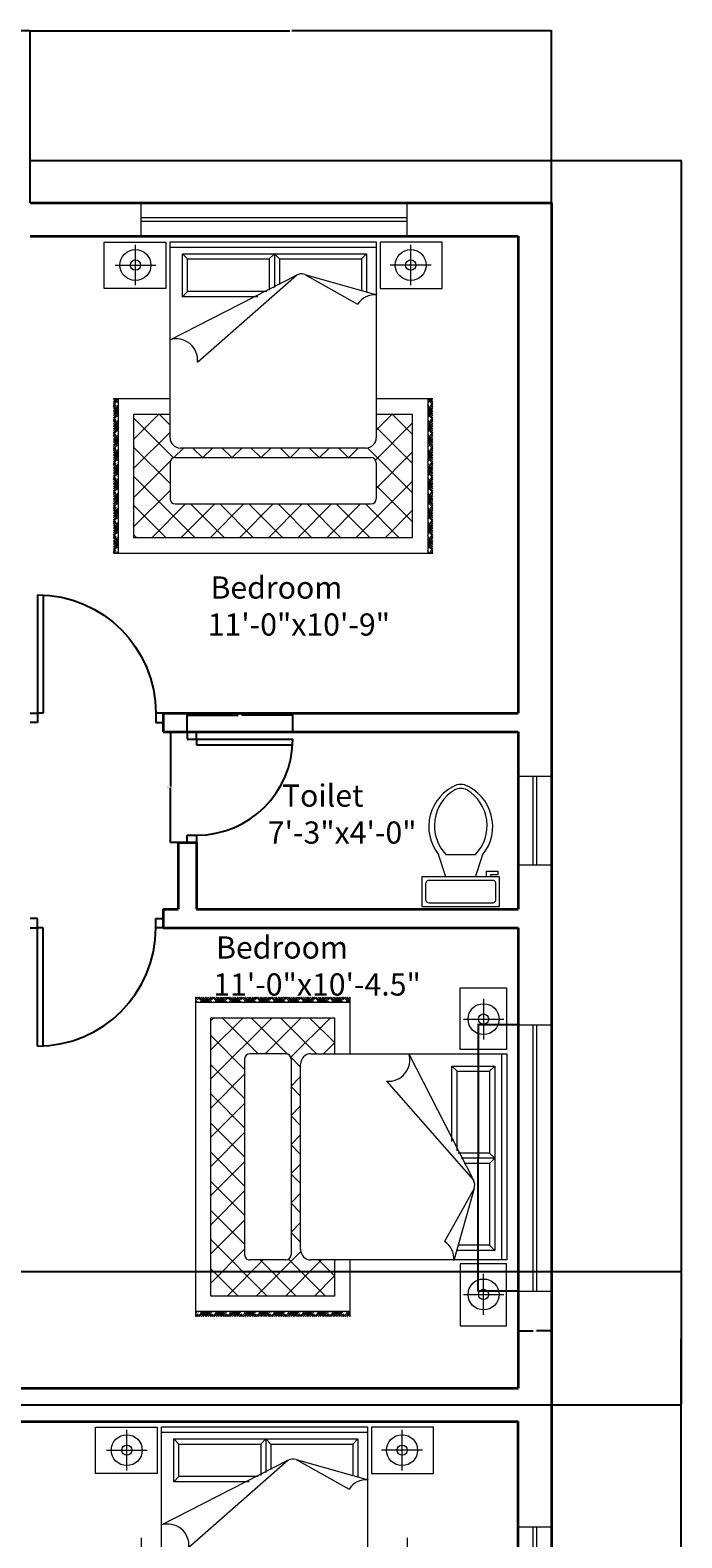
# Model space of a CAD drawing. Units: inches. Extents: x 3198 to 3702, y 1509 to 2253.
# Tile 6 of 6: x 3526 to 3702, y 1845 to 2253. Entities that reach past the tile are written whole.
import ezdxf

# ---------------------------------------------------------------- set-up
doc = ezdxf.new("R2010")
doc.units = ezdxf.units.IN
for name, color, linetype, lineweight in [('A-ANNO-DIMS', 2, 'Continuous', 18), ('A-AREA-IDEN', 7, 'Continuous', 18), ('A-DOOR', 3, 'Continuous', 25), ('A-FLOR-FIXT', 9, 'Continuous', 18), ('A-FURN', 8, 'Continuous', 13), ('A-GLAZ', 4, 'Continuous', 18), ('A-WALL', 7, 'Continuous', 35)]:
    doc.layers.add(name, color=color, linetype=linetype, lineweight=lineweight)
doc.styles.get("Standard").update_dxf_attribs({"font": 'arial.ttf'})
doc.dimstyles.get("Standard").update_dxf_attribs({"dimtxt": 0.18, "dimasz": 0.18, "dimexe": 0.18, "dimexo": 0.0625, "dimgap": 0.09, "dimtad": 0, "dimtih": 1, "dimtoh": 1, "dimdec": 4, "dimzin": 0, "dimdsep": 46, "dimtxsty": 'Standard', "dimcen": 0.09, "dimadec": 0, "dimazin": 0, "dimtfac": 1, "dimtdec": 4, "dimtofl": 0, "dimtmove": 0, "dimatfit": 3, "dimfxl": 1, "dimtolj": 1, "dimtzin": 0, "dimarcsym": 0})

# ---------------------------------------------------------------- blocks, each defined once
blk = doc.blocks.new('A$C4CB008C5')
for p, q in [((0, 3.019), (0.6, 3.019)), ((0, 2.569), (0, 3.019)), ((0.304, 2.6), (0.304, 2.992)), ((0.6, 3.019), (0.6, 2.569)), ((0.64, 1.121), (0.64, 3.021)), ((0.64, 3.021), (2.64, 3.021)), ((0.64, 2.971), (2.64, 2.971)), ((2.64, 3.021), (2.64, 1.121)), ((3.279, 3.019), (2.679, 3.019)), ((2.679, 3.019), (2.679, 2.569)), ((2.975, 2.6), (2.975, 2.992)), ((3.279, 2.569), (3.279, 3.019)), ((0.106, 2.796), (0.503, 2.796)), ((0.759, 2.905), (2.547, 2.905)), ((0.759, 2.489), (0.759, 2.905)), ((0.759, 2.905), (0.809, 2.855)), ((0.809, 2.855), (1.603, 2.855)), ((0.809, 2.539), (0.809, 2.855)), ((1.603, 2.855), (1.653, 2.905)), ((1.603, 2.855), (1.603, 2.551)), ((1.653, 2.905), (1.653, 2.579)), ((1.653, 2.905), (1.703, 2.855)), ((1.703, 2.855), (1.703, 2.607)), ((1.703, 2.855), (2.497, 2.855)), ((2.497, 2.855), (2.547, 2.905)), ((2.497, 2.855), (2.497, 2.556)), ((2.547, 2.905), (2.547, 2.54)), ((3.174, 2.796), (2.776, 2.796)), ((0.64, 2.071), (1.866, 2.698)), ((0.906, 1.854), (1.866, 2.698)), ((1.946, 2.705), (2.646, 2.507)), ((1.946, 2.705), (2.46, 2.418)), ((0.6, 2.569), (0, 2.569)), ((0.809, 2.539), (0.759, 2.489)), ((1.49, 2.489), (0.759, 2.489)), ((1.58, 2.539), (0.809, 2.539)), ((2.679, 2.569), (3.279, 2.569)), ((0.907, 1.867), (0.919, 1.867)), ((0.09, 1.5), (0.64, 1.5)), ((0.09, 1.491), (0.099, 1.5)), ((0.09, 1.473), (0.116, 1.5)), ((0.09, 1.456), (0.134, 1.5)), ((0.09, 1.474), (0.09, 1.475)), ((0.09, 1.438), (0.126, 1.474)), ((0.14, 1.46), (0.108, 1.492)), ((0.14, 1.478), (0.118, 1.5)), ((0.14, 1.496), (0.135, 1.5)), ((0.14, 0), (0.14, 1.5)), ((2.64, 1.5), (3.19, 1.5)), ((3.14, 1.496), (3.144, 1.5)), ((3.14, 1.478), (3.162, 1.5)), ((3.14, 1.5), (3.14, 0)), ((3.14, 1.46), (3.171, 1.492)), ((3.19, 1.456), (3.145, 1.5)), ((3.19, 1.438), (3.154, 1.474)), ((3.19, 1.473), (3.163, 1.5)), ((3.19, 1.491), (3.181, 1.5)), ((3.189, 1.474), (3.19, 1.475)), ((0.117, 1.43), (0.09, 1.457)), ((0.14, 1.389), (0.09, 1.439)), ((0.09, 1.42), (0.099, 1.43)), ((0.14, 1.372), (0.09, 1.422)), ((0.09, 1.368), (0.14, 1.417)), ((0.14, 1.354), (0.09, 1.404)), ((0.09, 1.35), (0.14, 1.4)), ((0.14, 1.336), (0.09, 1.386)), ((0.09, 1.332), (0.14, 1.382)), ((0.09, 1.314), (0.14, 1.364)), ((0.09, 1.297), (0.126, 1.333)), ((0.09, 1.333), (0.09, 1.333)), ((0.14, 1.319), (0.108, 1.35)), ((0.117, 1.412), (0.14, 1.435)), ((0.14, 1.442), (0.135, 1.448)), ((0.29, 1.108), (0.532, 1.35)), ((0.29, 0.15), (0.29, 1.35)), ((0.29, 1.35), (0.64, 1.35)), ((0.64, 1.243), (0.533, 1.35)), ((2.64, 1.195), (2.795, 1.35)), ((2.64, 1.35), (2.99, 1.35)), ((2.99, 1.156), (2.795, 1.35)), ((2.99, 1.35), (2.99, 0.15)), ((3.14, 1.442), (3.145, 1.448)), ((3.14, 1.389), (3.19, 1.439)), ((3.162, 1.412), (3.14, 1.435)), ((3.14, 1.372), (3.19, 1.422)), ((3.189, 1.368), (3.14, 1.417)), ((3.14, 1.354), (3.19, 1.404)), ((3.19, 1.35), (3.14, 1.4)), ((3.14, 1.336), (3.19, 1.386)), ((3.19, 1.332), (3.14, 1.382)), ((3.19, 1.314), (3.14, 1.364)), ((3.14, 1.319), (3.171, 1.35)), ((3.19, 1.297), (3.154, 1.333)), ((3.162, 1.43), (3.19, 1.457)), ((3.19, 1.42), (3.18, 1.43)), ((3.189, 1.333), (3.19, 1.333)), ((0.117, 1.288), (0.09, 1.316)), ((0.14, 1.248), (0.09, 1.298)), ((0.09, 1.279), (0.099, 1.288)), ((0.14, 1.23), (0.09, 1.28)), ((0.09, 1.227), (0.14, 1.276)), ((0.14, 1.213), (0.09, 1.263)), ((0.09, 1.208), (0.14, 1.258)), ((0.14, 1.195), (0.09, 1.245)), ((0.09, 1.19), (0.14, 1.24)), ((0.09, 1.173), (0.14, 1.223)), ((0.09, 1.191), (0.09, 1.192)), ((0.09, 1.155), (0.126, 1.191)), ((0.117, 1.147), (0.09, 1.174)), ((0.14, 1.177), (0.108, 1.209)), ((0.117, 1.271), (0.14, 1.294)), ((0.14, 1.301), (0.135, 1.306)), ((0.674, 0.926), (0.29, 1.31)), ((0.29, 0.825), (0.64, 1.175)), ((2.632, 0.904), (2.99, 1.262)), ((2.99, 0.873), (2.64, 1.223)), ((3.14, 1.301), (3.145, 1.306)), ((3.14, 1.248), (3.19, 1.298)), ((3.162, 1.271), (3.14, 1.294)), ((3.14, 1.23), (3.19, 1.28)), ((3.189, 1.227), (3.14, 1.276)), ((3.14, 1.213), (3.19, 1.263)), ((3.19, 1.208), (3.14, 1.258)), ((3.14, 1.195), (3.19, 1.245)), ((3.19, 1.19), (3.14, 1.24)), ((3.19, 1.173), (3.14, 1.223)), ((3.14, 1.177), (3.171, 1.209)), ((3.19, 1.155), (3.154, 1.191)), ((3.162, 1.288), (3.19, 1.316)), ((3.162, 1.147), (3.19, 1.174)), ((3.19, 1.279), (3.18, 1.288)), ((3.189, 1.191), (3.19, 1.192)), ((0.14, 1.107), (0.09, 1.157)), ((0.09, 1.137), (0.099, 1.147)), ((0.14, 1.089), (0.09, 1.139)), ((0.09, 1.085), (0.14, 1.134)), ((0.14, 1.071), (0.09, 1.121)), ((0.09, 1.067), (0.14, 1.117)), ((0.14, 1.054), (0.09, 1.104)), ((0.09, 1.049), (0.14, 1.099)), ((0.09, 1.031), (0.14, 1.081)), ((0.09, 1.05), (0.09, 1.051)), ((0.09, 1.014), (0.126, 1.05)), ((0.117, 1.006), (0.09, 1.033)), ((0.14, 1.036), (0.108, 1.067)), ((0.117, 1.129), (0.14, 1.152)), ((0.14, 1.16), (0.135, 1.165)), ((0.64, 0.677), (0.29, 1.027)), ((3.14, 1.16), (3.145, 1.165)), ((3.14, 1.107), (3.19, 1.157)), ((3.162, 1.129), (3.14, 1.152)), ((3.14, 1.089), (3.19, 1.139)), ((3.189, 1.085), (3.14, 1.134)), ((3.14, 1.071), (3.19, 1.121)), ((3.19, 1.067), (3.14, 1.117)), ((3.14, 1.054), (3.19, 1.104)), ((3.19, 1.049), (3.14, 1.099)), ((3.19, 1.031), (3.14, 1.081)), ((3.14, 1.036), (3.171, 1.067)), ((3.19, 1.014), (3.154, 1.05)), ((3.162, 1.006), (3.19, 1.033)), ((3.19, 1.137), (3.18, 1.147)), ((3.189, 1.05), (3.19, 1.051)), ((0.14, 0.965), (0.09, 1.015)), ((0.09, 0.996), (0.099, 1.006)), ((0.14, 0.948), (0.09, 0.998)), ((0.09, 0.944), (0.14, 0.993)), ((0.14, 0.93), (0.09, 0.98)), ((0.09, 0.925), (0.14, 0.975)), ((0.14, 0.912), (0.09, 0.962)), ((0.09, 0.908), (0.14, 0.958)), ((0.09, 0.89), (0.14, 0.94)), ((0.09, 0.908), (0.09, 0.909)), ((0.09, 0.872), (0.126, 0.908)), ((0.117, 0.864), (0.09, 0.891)), ((0.14, 0.894), (0.108, 0.926)), ((0.117, 0.988), (0.14, 1.011)), ((0.14, 1.018), (0.135, 1.023)), ((0.14, 0.877), (0.135, 0.882)), ((0.29, 0.542), (0.643, 0.895)), ((0.64, 0.878), (0.64, 0.528)), ((0.673, 0.925), (0.769, 1.021)), ((0.69, 0.928), (2.59, 0.928)), ((2.54, 1.021), (0.74, 1.021)), ((0.955, 0.928), (0.861, 1.021)), ((0.959, 0.928), (1.052, 1.021)), ((1.238, 0.928), (1.144, 1.021)), ((1.241, 0.928), (1.335, 1.021)), ((1.52, 0.928), (1.427, 1.021)), ((1.524, 0.928), (1.618, 1.021)), ((1.803, 0.928), (1.71, 1.021)), ((1.807, 0.928), (1.9, 1.021)), ((2.086, 0.928), (1.993, 1.021)), ((2.09, 0.928), (2.183, 1.021)), ((2.369, 0.928), (2.276, 1.021)), ((2.373, 0.928), (2.466, 1.021)), ((2.99, 0.59), (2.557, 1.023)), ((2.64, 0.629), (2.99, 0.979)), ((2.64, 0.878), (2.64, 0.528)), ((3.14, 1.018), (3.145, 1.023)), ((3.14, 0.965), (3.19, 1.015)), ((3.162, 0.988), (3.14, 1.011)), ((3.14, 0.948), (3.19, 0.998)), ((3.189, 0.944), (3.14, 0.993)), ((3.14, 0.93), (3.19, 0.98)), ((3.19, 0.925), (3.14, 0.975)), ((3.14, 0.912), (3.19, 0.962)), ((3.19, 0.908), (3.14, 0.958)), ((3.19, 0.89), (3.14, 0.94)), ((3.14, 0.894), (3.171, 0.926)), ((3.14, 0.877), (3.145, 0.882)), ((3.19, 0.872), (3.154, 0.908)), ((3.162, 0.864), (3.19, 0.891)), ((3.19, 0.996), (3.18, 1.006)), ((3.189, 0.908), (3.19, 0.909)), ((0.14, 0.824), (0.09, 0.874)), ((0.09, 0.855), (0.099, 0.864)), ((0.14, 0.806), (0.09, 0.856)), ((0.09, 0.802), (0.14, 0.852)), ((0.14, 0.788), (0.09, 0.838)), ((0.09, 0.784), (0.14, 0.834)), ((0.14, 0.771), (0.09, 0.821)), ((0.09, 0.766), (0.14, 0.816)), ((0.09, 0.749), (0.14, 0.799)), ((0.09, 0.767), (0.09, 0.768)), ((0.09, 0.731), (0.126, 0.767)), ((0.117, 0.723), (0.09, 0.75)), ((0.14, 0.682), (0.09, 0.732)), ((0.14, 0.753), (0.108, 0.785)), ((0.117, 0.847), (0.14, 0.869)), ((0.14, 0.735), (0.135, 0.74)), ((0.884, 0.15), (0.29, 0.744)), ((3.14, 0.824), (3.19, 0.874)), ((3.162, 0.847), (3.14, 0.869)), ((3.14, 0.806), (3.19, 0.856)), ((3.189, 0.802), (3.14, 0.852)), ((3.14, 0.788), (3.19, 0.838)), ((3.19, 0.784), (3.14, 0.834)), ((3.14, 0.771), (3.19, 0.821)), ((3.19, 0.766), (3.14, 0.816)), ((3.19, 0.749), (3.14, 0.799)), ((3.14, 0.753), (3.171, 0.785)), ((3.14, 0.735), (3.145, 0.74)), ((3.14, 0.682), (3.19, 0.732)), ((3.19, 0.731), (3.154, 0.767)), ((3.162, 0.723), (3.19, 0.75)), ((3.19, 0.855), (3.18, 0.864)), ((3.189, 0.767), (3.19, 0.768)), ((0.09, 0.713), (0.099, 0.723)), ((0.14, 0.665), (0.09, 0.715)), ((0.09, 0.661), (0.14, 0.71)), ((0.14, 0.647), (0.09, 0.697)), ((0.09, 0.642), (0.14, 0.692)), ((0.14, 0.629), (0.09, 0.679)), ((0.09, 0.625), (0.14, 0.675)), ((0.09, 0.607), (0.14, 0.657)), ((0.09, 0.589), (0.126, 0.626)), ((0.09, 0.626), (0.09, 0.626)), ((0.117, 0.581), (0.09, 0.609)), ((0.14, 0.541), (0.09, 0.591)), ((0.14, 0.612), (0.108, 0.643)), ((0.117, 0.705), (0.14, 0.728)), ((0.117, 0.564), (0.14, 0.586)), ((0.14, 0.594), (0.135, 0.599)), ((0.29, 0.259), (0.64, 0.609)), ((2.443, 0.15), (2.99, 0.696)), ((2.99, 0.307), (2.64, 0.657)), ((3.162, 0.705), (3.14, 0.728)), ((3.14, 0.665), (3.19, 0.715)), ((3.189, 0.661), (3.14, 0.71)), ((3.14, 0.647), (3.19, 0.697)), ((3.19, 0.642), (3.14, 0.692)), ((3.14, 0.629), (3.19, 0.679)), ((3.19, 0.625), (3.14, 0.675)), ((3.19, 0.607), (3.14, 0.657)), ((3.14, 0.612), (3.171, 0.643)), ((3.14, 0.594), (3.145, 0.599)), ((3.14, 0.541), (3.19, 0.591)), ((3.162, 0.564), (3.14, 0.586)), ((3.19, 0.589), (3.154, 0.626)), ((3.162, 0.581), (3.19, 0.609)), ((3.19, 0.713), (3.18, 0.723)), ((3.189, 0.626), (3.19, 0.626)), ((0.09, 0.572), (0.099, 0.581)), ((0.14, 0.523), (0.09, 0.573)), ((0.09, 0.519), (0.14, 0.569)), ((0.14, 0.506), (0.09, 0.556)), ((0.09, 0.501), (0.14, 0.551)), ((0.14, 0.488), (0.09, 0.538)), ((0.09, 0.483), (0.14, 0.533)), ((0.09, 0.466), (0.14, 0.516)), ((0.09, 0.484), (0.09, 0.485)), ((0.09, 0.448), (0.126, 0.484)), ((0.117, 0.44), (0.09, 0.467)), ((0.14, 0.399), (0.09, 0.449)), ((0.09, 0.43), (0.099, 0.44)), ((0.14, 0.47), (0.108, 0.502)), ((0.117, 0.422), (0.14, 0.445)), ((0.14, 0.453), (0.135, 0.458)), ((0.601, 0.15), (0.29, 0.462)), ((0.463, 0.15), (0.791, 0.478)), ((0.69, 0.478), (2.59, 0.478)), ((0.746, 0.15), (1.074, 0.478)), ((1.167, 0.15), (0.839, 0.478)), ((1.029, 0.15), (1.357, 0.478)), ((1.45, 0.15), (1.122, 0.478)), ((1.312, 0.15), (1.64, 0.478)), ((1.733, 0.15), (1.405, 0.478)), ((1.595, 0.15), (1.923, 0.478)), ((2.016, 0.15), (1.688, 0.478)), ((1.878, 0.15), (2.206, 0.478)), ((2.298, 0.15), (1.97, 0.478)), ((2.16, 0.15), (2.488, 0.478)), ((2.581, 0.15), (2.253, 0.478)), ((2.864, 0.15), (2.536, 0.478)), ((3.14, 0.523), (3.19, 0.573)), ((3.189, 0.519), (3.14, 0.569)), ((3.14, 0.506), (3.19, 0.556)), ((3.19, 0.501), (3.14, 0.551)), ((3.14, 0.488), (3.19, 0.538)), ((3.19, 0.483), (3.14, 0.533)), ((3.19, 0.466), (3.14, 0.516)), ((3.14, 0.47), (3.171, 0.502)), ((3.14, 0.453), (3.145, 0.458)), ((3.14, 0.399), (3.19, 0.449)), ((3.162, 0.422), (3.14, 0.445)), ((3.19, 0.448), (3.154, 0.484)), ((3.162, 0.44), (3.19, 0.467)), ((3.19, 0.572), (3.18, 0.581)), ((3.19, 0.43), (3.18, 0.44)), ((3.189, 0.484), (3.19, 0.485)), ((0.14, 0.382), (0.09, 0.432)), ((0.09, 0.378), (0.14, 0.427)), ((0.14, 0.364), (0.09, 0.414)), ((0.09, 0.36), (0.14, 0.41)), ((0.14, 0.346), (0.09, 0.396)), ((0.09, 0.342), (0.14, 0.392)), ((0.09, 0.324), (0.14, 0.374)), ((0.09, 0.307), (0.126, 0.343)), ((0.09, 0.343), (0.09, 0.343)), ((0.117, 0.299), (0.09, 0.326)), ((0.14, 0.258), (0.09, 0.308)), ((0.09, 0.289), (0.099, 0.299)), ((0.14, 0.329), (0.108, 0.36)), ((0.117, 0.281), (0.14, 0.304)), ((0.14, 0.311), (0.135, 0.316)), ((2.726, 0.15), (2.99, 0.414)), ((3.14, 0.382), (3.19, 0.432)), ((3.189, 0.378), (3.14, 0.427)), ((3.14, 0.364), (3.19, 0.414)), ((3.19, 0.36), (3.14, 0.41)), ((3.14, 0.346), (3.19, 0.396)), ((3.19, 0.342), (3.14, 0.392)), ((3.19, 0.324), (3.14, 0.374)), ((3.14, 0.329), (3.171, 0.36)), ((3.14, 0.311), (3.145, 0.316)), ((3.14, 0.258), (3.19, 0.308)), ((3.162, 0.281), (3.14, 0.304)), ((3.19, 0.307), (3.154, 0.343)), ((3.162, 0.299), (3.19, 0.326)), ((3.19, 0.289), (3.18, 0.299)), ((3.189, 0.343), (3.19, 0.343)), ((0.14, 0.24), (0.09, 0.29)), ((0.09, 0.237), (0.14, 0.286)), ((0.14, 0.223), (0.09, 0.273)), ((0.09, 0.218), (0.14, 0.268)), ((0.14, 0.205), (0.09, 0.255)), ((0.09, 0.201), (0.14, 0.251)), ((0.09, 0.183), (0.14, 0.233)), ((0.09, 0.201), (0.09, 0.202)), ((0.09, 0.165), (0.126, 0.201)), ((0.117, 0.157), (0.09, 0.184)), ((0.14, 0.117), (0.09, 0.167)), ((0.09, 0.148), (0.099, 0.157)), ((0.14, 0.099), (0.09, 0.149)), ((0.14, 0.187), (0.108, 0.219)), ((0.117, 0.139), (0.14, 0.162)), ((0.14, 0.17), (0.135, 0.175)), ((0.318, 0.15), (0.29, 0.179)), ((2.99, 0.15), (0.29, 0.15)), ((3.14, 0.24), (3.19, 0.29)), ((3.189, 0.237), (3.14, 0.286)), ((3.14, 0.223), (3.19, 0.273)), ((3.19, 0.218), (3.14, 0.268)), ((3.14, 0.205), (3.19, 0.255)), ((3.19, 0.201), (3.14, 0.251)), ((3.19, 0.183), (3.14, 0.233)), ((3.14, 0.187), (3.171, 0.219)), ((3.14, 0.17), (3.145, 0.175)), ((3.14, 0.117), (3.19, 0.167)), ((3.162, 0.139), (3.14, 0.162)), ((3.14, 0.099), (3.19, 0.149)), ((3.19, 0.165), (3.154, 0.201)), ((3.162, 0.157), (3.19, 0.184)), ((3.19, 0.148), (3.18, 0.157)), ((3.189, 0.201), (3.19, 0.202)), ((0.09, 0.095), (0.14, 0.144)), ((0.14, 0.081), (0.09, 0.131)), ((0.09, 0.077), (0.14, 0.127)), ((0.14, 0.064), (0.09, 0.114)), ((0.09, 0.059), (0.14, 0.109)), ((0.09, 0.041), (0.14, 0.091)), ((0.09, 0.06), (0.09, 0.061)), ((0.09, 0.024), (0.126, 0.06)), ((0.117, 0.016), (0.09, 0.043)), ((0.115, 0), (0.09, 0.025)), ((0.09, 0.006), (0.099, 0.016)), ((0.097, 0), (0.09, 0.008)), ((0.14, 0.046), (0.108, 0.078)), ((0.119, 0), (0.14, 0.021)), ((0.14, 0.028), (0.135, 0.033)), ((0.137, 0), (0.14, 0.003)), ((3.189, 0.095), (3.14, 0.144)), ((3.14, 0.081), (3.19, 0.131)), ((3.19, 0.077), (3.14, 0.127)), ((3.14, 0.064), (3.19, 0.114)), ((3.19, 0.059), (3.14, 0.109)), ((3.19, 0.041), (3.14, 0.091)), ((3.14, 0.046), (3.171, 0.078)), ((3.14, 0.028), (3.145, 0.033)), ((3.16, 0), (3.14, 0.021)), ((3.143, 0), (3.14, 0.003)), ((3.19, 0.024), (3.154, 0.06)), ((3.162, 0.016), (3.19, 0.043)), ((3.164, 0), (3.19, 0.025)), ((3.19, 0.006), (3.18, 0.016)), ((3.182, 0), (3.19, 0.008)), ((3.189, 0.06), (3.19, 0.061)), ((0.09, 0), (3.19, 0))]:
    blk.add_line(p, q)
for centre, radius in [((0.304, 2.796), 0.15), ((2.975, 2.796), 0.15), ((0.304, 2.796), 0.05), ((2.975, 2.796), 0.05)]:
    blk.add_circle(centre, radius)
for centre, radius, start, end in [((1.915, 2.61), 0.1, 71.7215, 119.0799), ((2.626, 2.31), 0.198, 84.1725, 146.9889), ((0.7, 1.873), 0.207, 354.6422, 106.9775), ((0.74, 1.121), 0.1, 180, 270), ((2.54, 1.121), 0.1, 270, 0), ((0.69, 0.878), 0.05, 90, 180), ((2.59, 0.878), 0.05, 0, 90), ((0.69, 0.528), 0.05, 180, 270), ((2.59, 0.528), 0.05, 270, 0)]:
    blk.add_arc(centre, radius, start, end)
blk = doc.blocks.new('*U4')
for p, q in [((9.5, -6), (9.5, -2)), ((-8, -8.5), (-8, -8)), ((-7, -8), (-7, -9.5)), ((-4, -8), (-6, -14)), ((4, -8), (6, -14)), ((-10, -8.5), (-8, -8.5)), ((-10, -9.5), (-10, -8.5)), ((-7, -9.5), (-10, -9.5)), ((4, -14), (-4, -14))]:
    blk.add_line(p, q)
blk.add_lwpolyline([(10.5, -8), (10.5, 0), (-10.5, 0), (-10.5, -8)], close=True)
for points in [[(-9.5, -2), (-9.5, -6)], [(8.5, -1), (-8.5, -1)], [(-8.5, -7), (8.5, -7)]]:
    blk.add_lwpolyline(points)
for centre, radius, start, end in [((-8.62, -1.88), 0.884, 81.8699, 188.1301), ((8.62, -1.88), 0.884, 351.8699, 98.1301), ((-8.62, -6.12), 0.884, 171.8699, 278.1301), ((8.62, -6.12), 0.884, 261.8699, 8.1301), ((3.52, -21.58), 12.17, 141.4691, 247.9714), ((4.2, -21.82), 11.33, 136.3677, 238.9468), ((-3.52, -21.58), 12.17, 292.0284, 38.5307), ((-4.2, -21.82), 11.33, 301.053, 43.6321), ((0, -27.88), 4, 245.7318, 294.2682), ((0, -29), 4, 254.8605, 285.1395)]:
    blk.add_arc(centre, radius, start, end)
blk = doc.blocks.new('DOOR-SINGLE-32')
for p, q in [((0, 34), (32, 34)), ((32, 36), (32, 34)), ((32, 34), (34.5, 34)), ((32, 32.5), (32, 34)), ((34.5, 34), (34.5, 36)), ((0.04, 32.5), (32, 32.5)), ((32, 0), (32, 2)), ((32, 2), (34.5, 2)), ((34.5, 2), (34.5, 0))]:
    blk.add_line(p, q)
blk.add_arc((32, 34), 32, 180, 270)
blk = doc.blocks.new('DOOR-SINGLE-26')
for p, q in [((0, 30), (0, 28)), ((2.5, 28), (2.5, 30)), ((0, 28), (2.5, 28)), ((2.5, 28), (28.5, 28)), ((2.5, 28), (2.5, 26.5)), ((2.5, 26.5), (28.46, 26.5)), ((0, 0), (0, 2)), ((0, 2), (2.5, 2)), ((2.5, 2), (2.5, 0))]:
    blk.add_line(p, q)
blk.add_arc((2.5, 28), 26, 270, 0)
blk = doc.blocks.new('WIN-72-W9')
for p, q in [((0, 0), (0, 9)), ((72, 0), (72, 9)), ((72, 5), (0, 5)), ((72, 4), (0, 4))]:
    blk.add_line(p, q)
blk = doc.blocks.new('WIN-24-W9')
for p, q in [((9, 24), (0, 24)), ((4, 24), (4, 0)), ((5, 24), (5, 0)), ((9, 0), (0, 0))]:
    blk.add_line(p, q)
blk = doc.blocks.new('*D17')
at = {"layer": 'A-ANNO-DIMS', "color": 0, "lineweight": -2, "transparency": 16777216}
for p, q in [((3657.48, 1983.64), (3646.57, 1983.64)), ((3646.75, 1983.46), (3646.75, 1947.82)), ((3646.75, 1911.82), (3646.75, 1947.45)), ((3657.48, 1911.64), (3646.57, 1911.64))]:
    blk.add_line(p, q, dxfattribs=at)
at = {"layer": 'A-ANNO-DIMS', "color": 0, "transparency": 16777216}
for points in [[(3646.72, 1983.46), (3646.78, 1983.46), (3646.75, 1983.64)], [(3646.72, 1911.82), (3646.78, 1911.82), (3646.75, 1911.64)]]:
    blk.add_solid(points, dxfattribs=at)
at = {"layer": 'Defpoints', "color": 0, "transparency": 16777216}
for p in [(3657.55, 1983.64), (3646.75, 1911.64), (3657.55, 1911.64)]:
    blk.add_point(p, dxfattribs=at)
at = {"layer": 'A-ANNO-DIMS', "color": 0, "transparency": 16777216, "insert": (3646.75, 1947.64), "char_height": 0.18, "attachment_point": 5}
blk.add_mtext('\\A1;WINDOW 72 TYP.', dxfattribs=at)
blk = doc.blocks.new('*D18')
at = {"layer": 'A-ANNO-DIMS', "color": 0, "lineweight": -2, "transparency": 16777216}
for p, q in [((3657.55, 1911.58), (3657.55, 1900.66)), ((3666.55, 1911.58), (3666.55, 1900.66)), ((3657.73, 1900.84), (3661.59, 1900.84)), ((3666.37, 1900.84), (3662.51, 1900.84))]:
    blk.add_line(p, q, dxfattribs=at)
at = {"layer": 'A-ANNO-DIMS', "color": 0, "transparency": 16777216}
for points in [[(3657.73, 1900.87), (3657.73, 1900.81), (3657.55, 1900.84)], [(3666.37, 1900.87), (3666.37, 1900.81), (3666.55, 1900.84)]]:
    blk.add_solid(points, dxfattribs=at)
at = {"layer": 'Defpoints', "color": 0, "transparency": 16777216}
for p in [(3657.55, 1911.64), (3666.55, 1911.64), (3666.55, 1900.84)]:
    blk.add_point(p, dxfattribs=at)
at = {"layer": 'A-ANNO-DIMS', "color": 0, "transparency": 16777216, "insert": (3662.05, 1900.84), "char_height": 0.18, "attachment_point": 5}
blk.add_mtext('\\A1;9 TYP.', dxfattribs=at)
blk = doc.blocks.new('*D23')
at = {"layer": 'A-ANNO-DIMS', "color": 0, "lineweight": -2, "transparency": 16777216}
for p, q in [((3567.98, 2062.89), (3563.37, 2062.89)), ((3563.55, 2062.71), (3563.55, 2048.07)), ((3563.55, 2033.07), (3563.55, 2047.7)), ((3567.98, 2032.89), (3563.37, 2032.89))]:
    blk.add_line(p, q, dxfattribs=at)
at = {"layer": 'A-ANNO-DIMS', "color": 0, "transparency": 16777216}
for points in [[(3563.52, 2062.71), (3563.58, 2062.71), (3563.55, 2062.89)], [(3563.52, 2033.07), (3563.58, 2033.07), (3563.55, 2032.89)]]:
    blk.add_solid(points, dxfattribs=at)
at = {"layer": 'Defpoints', "color": 0, "transparency": 16777216}
for p in [(3563.55, 2062.89), (3568.05, 2062.89), (3568.05, 2032.89)]:
    blk.add_point(p, dxfattribs=at)
at = {"layer": 'A-ANNO-DIMS', "color": 0, "transparency": 16777216, "insert": (3563.55, 2047.89), "char_height": 0.18, "attachment_point": 5}
blk.add_mtext('\\A1;WC DOOR 30 TYP.', dxfattribs=at)
blk = doc.blocks.new('*D24')
at = {"layer": 'A-ANNO-DIMS', "color": 0, "lineweight": -2, "transparency": 16777216}
for p, q in [((3568.05, 2062.95), (3568.05, 2067.57)), ((3568.23, 2067.39), (3581.77, 2067.39)), ((3596.37, 2067.39), (3582.83, 2067.39)), ((3596.55, 2062.95), (3596.55, 2067.57))]:
    blk.add_line(p, q, dxfattribs=at)
at = {"layer": 'A-ANNO-DIMS', "color": 0, "transparency": 16777216}
for points in [[(3568.23, 2067.42), (3568.23, 2067.36), (3568.05, 2067.39)], [(3596.37, 2067.42), (3596.37, 2067.36), (3596.55, 2067.39)]]:
    blk.add_solid(points, dxfattribs=at)
at = {"layer": 'Defpoints', "color": 0, "transparency": 16777216}
for p in [(3596.55, 2067.39), (3568.05, 2062.89), (3596.55, 2062.89)]:
    blk.add_point(p, dxfattribs=at)
at = {"layer": 'A-ANNO-DIMS', "color": 0, "transparency": 16777216, "insert": (3582.3, 2067.39), "char_height": 0.18, "attachment_point": 5}
blk.add_mtext('\\A1;29 TYP.', dxfattribs=at)
blk = doc.blocks.new('*D44')
at = {"layer": 'A-ANNO-DIMS', "color": 0, "lineweight": -2, "transparency": 16777216}
for p, q in [((3525.61, 2217.39), (3701.78, 2217.39)), ((3701.6, 2217.21), (3701.6, 1881.07)), ((3701.6, 1544.57), (3701.6, 1880.71)), ((3525.61, 1544.39), (3701.78, 1544.39))]:
    blk.add_line(p, q, dxfattribs=at)
at = {"layer": 'A-ANNO-DIMS', "color": 0, "transparency": 16777216}
for points in [[(3701.57, 2217.21), (3701.63, 2217.21), (3701.6, 2217.39)], [(3701.57, 1544.57), (3701.63, 1544.57), (3701.6, 1544.39)]]:
    blk.add_solid(points, dxfattribs=at)
at = {"layer": 'Defpoints', "color": 0, "transparency": 16777216}
for p in [(3525.55, 2217.39), (3701.6, 2217.39), (3525.55, 1544.39)]:
    blk.add_point(p, dxfattribs=at)
at = {"layer": 'A-ANNO-DIMS', "color": 0, "transparency": 16777216, "insert": (3701.6, 1880.89), "char_height": 0.18, "attachment_point": 5}
blk.add_mtext('\\A1;673', dxfattribs=at)
blk = doc.blocks.new('*D46')
at = {"layer": 'A-ANNO-DIMS', "color": 0, "lineweight": -2, "transparency": 16777216}
for p, q in [((3383.55, 2217.45), (3383.55, 2252.62)), ((3383.73, 2252.44), (3454.27, 2252.44)), ((3525.37, 2252.44), (3454.83, 2252.44)), ((3525.55, 2217.45), (3525.55, 2252.62))]:
    blk.add_line(p, q, dxfattribs=at)
at = {"layer": 'A-ANNO-DIMS', "color": 0, "transparency": 16777216}
for points in [[(3383.73, 2252.47), (3383.73, 2252.41), (3383.55, 2252.44)], [(3525.37, 2252.47), (3525.37, 2252.41), (3525.55, 2252.44)]]:
    blk.add_solid(points, dxfattribs=at)
at = {"layer": 'Defpoints', "color": 0, "transparency": 16777216}
for p in [(3525.55, 2252.44), (3383.55, 2217.39), (3525.55, 2217.39)]:
    blk.add_point(p, dxfattribs=at)
at = {"layer": 'A-ANNO-DIMS', "color": 0, "transparency": 16777216, "insert": (3454.55, 2252.44), "char_height": 0.18, "attachment_point": 5}
blk.add_mtext('\\A1;142', dxfattribs=at)
blk = doc.blocks.new('*D47')
at = {"layer": 'A-ANNO-DIMS', "color": 0, "lineweight": -2, "transparency": 16777216}
for p, q in [((3525.55, 2205.95), (3525.55, 2252.62)), ((3525.73, 2252.44), (3595.78, 2252.44)), ((3666.37, 2252.44), (3596.31, 2252.44)), ((3666.55, 2205.95), (3666.55, 2252.62))]:
    blk.add_line(p, q, dxfattribs=at)
at = {"layer": 'A-ANNO-DIMS', "color": 0, "transparency": 16777216}
for points in [[(3525.73, 2252.47), (3525.73, 2252.41), (3525.55, 2252.44)], [(3666.37, 2252.47), (3666.37, 2252.41), (3666.55, 2252.44)]]:
    blk.add_solid(points, dxfattribs=at)
at = {"layer": 'Defpoints', "color": 0, "transparency": 16777216}
for p in [(3666.55, 2252.44), (3525.55, 2205.89), (3666.55, 2205.89)]:
    blk.add_point(p, dxfattribs=at)
at = {"layer": 'A-ANNO-DIMS', "color": 0, "transparency": 16777216, "insert": (3596.05, 2252.44), "char_height": 0.18, "attachment_point": 5}
blk.add_mtext('\\A1;141', dxfattribs=at)
blk = doc.blocks.new('*D55')
at = {"layer": 'A-ANNO-DIMS', "color": 0, "lineweight": -2, "transparency": 16777216}
for p, q in [((3383.61, 1916.89), (3701.78, 1916.89)), ((3701.6, 1916.71), (3701.6, 1899.07)), ((3701.6, 1881.07), (3701.6, 1898.71)), ((3383.61, 1880.89), (3701.78, 1880.89))]:
    blk.add_line(p, q, dxfattribs=at)
at = {"layer": 'A-ANNO-DIMS', "color": 0, "transparency": 16777216}
for points in [[(3701.57, 1916.71), (3701.63, 1916.71), (3701.6, 1916.89)], [(3701.57, 1881.07), (3701.63, 1881.07), (3701.6, 1880.89)]]:
    blk.add_solid(points, dxfattribs=at)
at = {"layer": 'Defpoints', "color": 0, "transparency": 16777216}
for p in [(3383.55, 1916.89), (3701.6, 1916.89), (3383.55, 1880.89)]:
    blk.add_point(p, dxfattribs=at)
at = {"layer": 'A-ANNO-DIMS', "color": 0, "transparency": 16777216, "insert": (3701.6, 1898.89), "char_height": 0.18, "attachment_point": 5}
blk.add_mtext('\\A1;36', dxfattribs=at)

msp = doc.modelspace()

# ---------------------------------------------------------------- linework, layer by layer
at = {"layer": 'A-WALL'}
for p, q in [((3525.5475, 2205.888), (3666.5475, 2205.888)), ((3666.5475, 2205.888), (3666.5475, 1555.888)), ((3525.5475, 2196.888), (3657.5475, 2196.888)), ((3657.5475, 2196.888), (3657.5475, 2067.888)), ((3561.5475, 2067.888), (3657.5475, 2067.888)), ((3561.5475, 2067.888), (3561.5475, 2062.888)), ((3561.5475, 2062.888), (3657.5475, 2062.888)), ((3657.5475, 2062.888), (3657.5475, 2014.888)), ((3565.5475, 2032.888), (3565.5475, 2014.888)), ((3565.5475, 2032.888), (3570.5475, 2032.888)), ((3570.5475, 2032.888), (3570.5475, 2014.888)), ((3561.5475, 2014.888), (3561.5475, 2009.888)), ((3561.5475, 2014.888), (3565.5475, 2014.888)), ((3570.5475, 2014.888), (3657.5475, 2014.888)), ((3561.5475, 2009.888), (3657.5475, 2009.888)), ((3657.5475, 2009.888), (3657.5475, 1885.388)), ((3513.5475, 1885.388), (3657.5475, 1885.388)), ((3513.5475, 1876.388), (3657.5475, 1876.388)), ((3657.5475, 1747.388), (3657.5475, 1876.388))]:
    msp.add_line(p, q, dxfattribs=at)

# ---------------------------------------------------------------- block references
at = {"layer": 'A-DOOR', "extrusion": (0, 0, -1), "zscale": -1, "rotation": 269.9999999999991}
msp.add_blockref('DOOR-SINGLE-32', (-3561.5475, 2099.8885), dxfattribs=at)
at = {"layer": 'A-DOOR'}
msp.add_blockref('DOOR-SINGLE-26', (3568.047, 2032.888), dxfattribs=at)
at = {"layer": 'A-DOOR', "rotation": 89.99999999999925}
msp.add_blockref('DOOR-SINGLE-32', (3561.5475, 1977.8875), dxfattribs=at)
at = {"layer": 'A-FLOR-FIXT', "rotation": 180}
msp.add_blockref('*U4', (3642.0095, 2015.6602), dxfattribs=at)
at = {"layer": 'A-FURN', "xscale": 27.87562936897135, "yscale": 27.87562936897135, "zscale": 27.87562936897135}
for p in [(3545.5496, 2111.157), (3543.2133, 1790.657)]:
    msp.add_blockref('A$C4CB008C5', p, dxfattribs=at)
at = {"layer": 'A-FURN', "xscale": 27.87562936897135, "yscale": 27.87562936897135, "zscale": 27.87562936897135, "rotation": 270}
msp.add_blockref('A$C4CB008C5', (3570.2384, 1993.6355), dxfattribs=at)
at = {"layer": 'A-GLAZ'}
msp.add_blockref('WIN-72-W9', (3555.547, 2196.888), dxfattribs=at)
for name, p, rotation in [('WIN-24-W9', (3666.5479, 2050.888), 180), ('WIN-72-W9', (3657.5475, 1983.6385), 270), ('WIN-72-W9', (3657.5475, 1847.8885), 270.0000000000002), ('WIN-72-W9', (3627.5479, 1844.888), 180)]:
    msp.add_blockref(name, p, dxfattribs=dict(at, rotation=rotation))

# ---------------------------------------------------------------- texts
at = {"layer": 'A-AREA-IDEN', "char_height": 2.5, "attachment_point": 1}
for s, insert in [(' {\\H2.4x;Bedroom\\P11\'-0"x10\'-9"}', (3573.56, 2104.8876)), ('     {\\H2.4x;Toilet\\P7\'-3"x4\'-0"}', (3589.8162, 2048.6234)), (' {\\H2.4x;Bedroom\\P11\'-0"x10\'-4.5"}', (3575.0691, 2007.5421))]:
    msp.add_mtext_dynamic_manual_height_columns(s, width=40.568847, gutter_width=12.5, heights=[0], dxfattribs=dict(at, insert=insert))

# ---------------------------------------------------------------- dimensions: what is measured, and where the dimension line sits
at = {"layer": 'A-ANNO-DIMS'}
for base, p1, p2, picture, middle in [((3525.5475, 2252.438), (3383.5475, 2217.388), (3525.5475, 2217.388), '*D46', (3454.5475, 2252.438)), ((3666.5475, 2252.438), (3525.5475, 2205.888), (3666.5475, 2205.888), '*D47', (3596.0475, 2252.438))]:
    dim = msp.add_linear_dim(base=base, p1=p1, p2=p2, dimstyle='Standard', override={"dimdec": 0, "dimlfac": 1, "dimrnd": 0, "dimzin": 0, "dimdsep": 46, "dimlunit": 2}, dxfattribs=at)
    dim.commit()
    dim.dimension.update_dxf_attribs({"geometry": picture, "text_midpoint": middle})
for base, p1, p2, picture, middle in [((3701.5975, 2217.388), (3525.5475, 1544.388), (3525.5475, 2217.388), '*D44', (3701.5975, 1880.888)), ((3701.5975, 1916.888), (3383.5475, 1880.888), (3383.5475, 1916.888), '*D55', (3701.5975, 1898.888))]:
    dim = msp.add_linear_dim(base=base, p1=p1, p2=p2, angle=90, dimstyle='Standard', override={"dimdec": 0, "dimlfac": 1, "dimrnd": 0, "dimzin": 0, "dimdsep": 46, "dimlunit": 2}, dxfattribs=at)
    dim.commit()
    dim.dimension.update_dxf_attribs({"geometry": picture, "text_midpoint": middle})
for base, p1, p2, picture, middle in [((3596.5474569853, 2067.3880023156), (3568.0474569853, 2062.8880023156), (3596.5474569853, 2062.8880023156), '*D24', (3582.2974569853, 2067.3880023156)), ((3666.5475, 1900.838), (3657.5475, 1911.638), (3666.5475, 1911.638), '*D18', (3662.0475, 1900.838))]:
    dim = msp.add_linear_dim(base=base, p1=p1, p2=p2, text='<> TYP.', dimstyle='Standard', override={"dimdec": 0, "dimlfac": 1, "dimrnd": 0, "dimzin": 0, "dimdsep": 46, "dimlunit": 2}, dxfattribs=at)
    dim.commit()
    dim.dimension.update_dxf_attribs({"geometry": picture, "text_midpoint": middle})
for base, p1, p2, angle, text, picture, middle in [((3563.5475, 2062.888), (3568.0475, 2032.888), (3568.0475, 2062.888), 90, 'WC DOOR <> TYP.', '*D23', (3563.5475, 2047.888)), ((3646.7475, 1911.638), (3657.5475, 1983.638), (3657.5475, 1911.638), 270, 'WINDOW <> TYP.', '*D17', (3646.7475, 1947.638))]:
    dim = msp.add_linear_dim(base=base, p1=p1, p2=p2, angle=angle, text=text, dimstyle='Standard', override={"dimdec": 0, "dimlfac": 1, "dimrnd": 0, "dimzin": 0, "dimdsep": 46, "dimlunit": 2}, dxfattribs=at)
    dim.commit()
    dim.dimension.update_dxf_attribs({"geometry": picture, "text_midpoint": middle})

doc.saveas('drawing.dxf')
